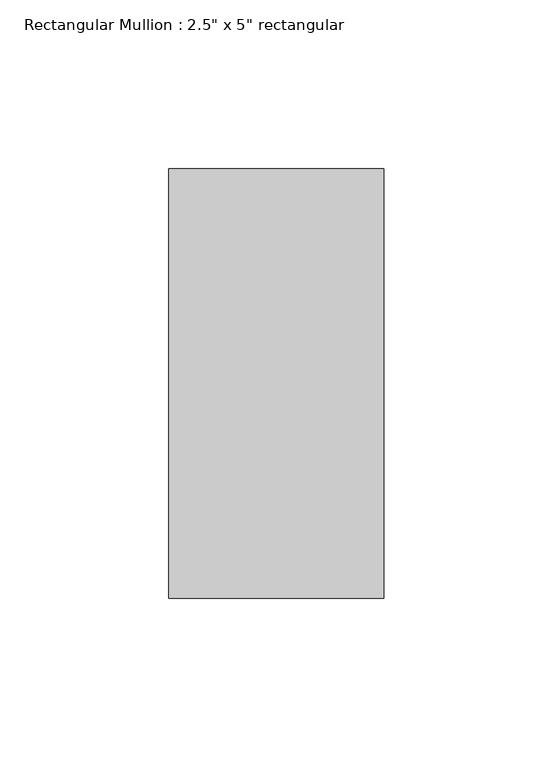
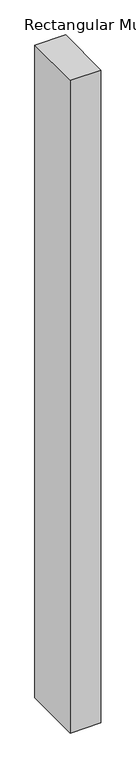
"""IFC4 building model written with IfcOpenShell, lengths in millimetres: member geometry."""

from ifc_helpers import new_model, si_unit, frame, origin, place, context, project, spatial, polyline, outline, extrude, source, transform, mapped, element, save


def member_7ec67256(model_context):
    return source(origin(), model_context, "Body", "SweptSolid", [
        extrude(outline(polyline([(0.0, 63.5), (0.0, -63.5), (-63.5, -63.5), (-63.5, 63.5), (0.0, 63.5)])), frame((0.0, 0.0, -1429.9871892), z_axis=(0.0, 0.0, 1.0), x_axis=(1.0, 0.0, 0.0)), (0.0, 0.0, 1.0), 1429.9871892),
    ])


if __name__ == "__main__":
    model = new_model("IFC4")
    model_context = context("Model", 3, world=origin())
    ifc_project = project(units=[si_unit("LENGTHUNIT", "METRE", prefix="MILLI")], contexts=[model_context])
    site = spatial("IfcSite", under=ifc_project)
    building = spatial("IfcBuilding", under=site)
    placement = place(None, origin())
    member_shape = member_7ec67256(model_context)
    element("IfcMember", 1, ObjectType="Rectangular Mullion : 2.5\" x 5\" rectangular", at=placement, inside=building, context=model_context, shape_type="MappedRepresentation", body=[
        mapped(member_shape, transform((0.0, 0.0, 0.0), x_axis=(1.0, 0.0, 0.0), y_axis=(0.0, 1.0, 0.0), z_axis=(0.0, 0.0, 1.0))),
    ])
    save(model, "model.ifc")

# Revit data of these elements
# Type "Rectangular Mullion : 2.5\" x 5\" rectangular"
#   built-in parameter 1007304 = 0.416667 (stored number, unit not read)
#   built-in parameter 1007301 = 0.104167 (stored number, unit not read)
#   built-in parameter 1007300 = 0.104167 (stored number, unit not read)
# Element 1 (IfcMember, "Rectangular Mullion : 2.5\" x 5\" rectangular")
#   Materials on its faces: "Aluminum"
# Materials
#   "Aluminum": class "Metal", colour RGB 247 247 247, transparency 0, Description = "Aluminum 6061", Cost = 0
